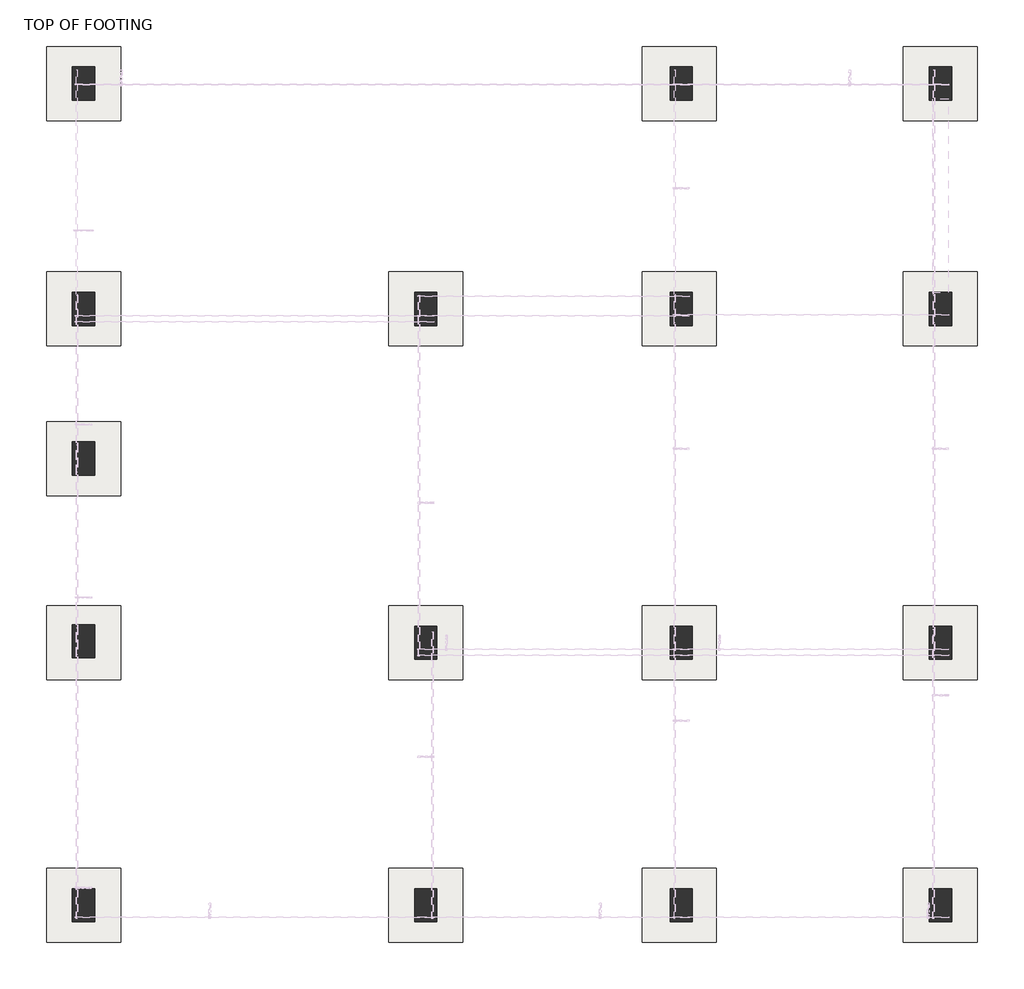
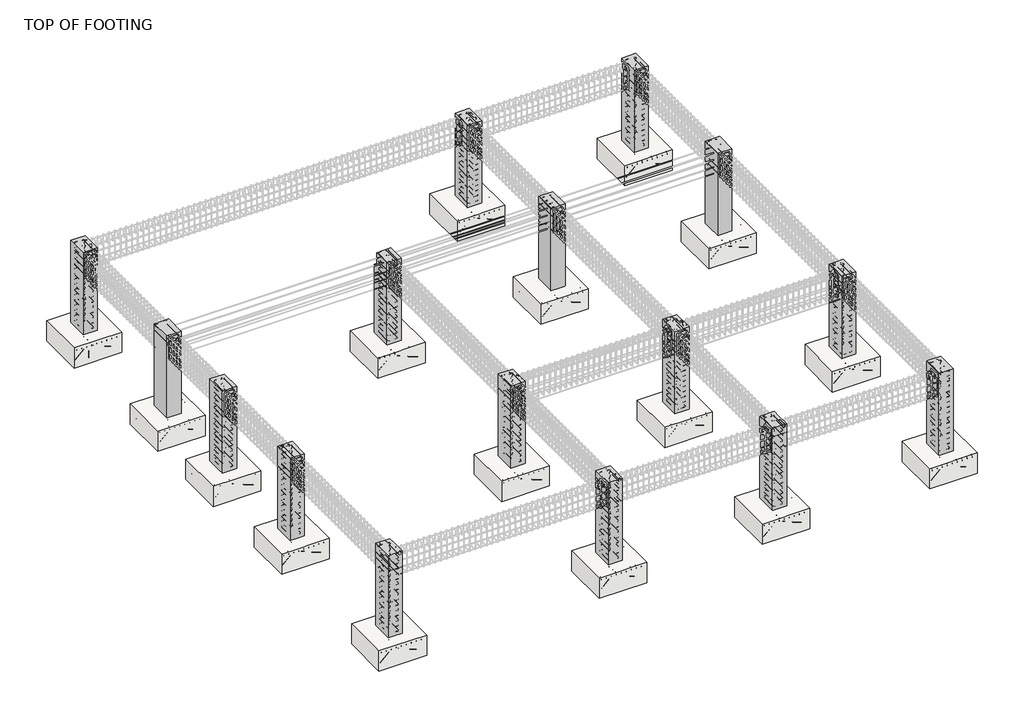
# One storey, part 1 of 13: 16 columns, 16 slabs.
"""IFC4 building model written with IfcOpenShell, lengths in millimetres."""

from ifc_helpers import new_model, si_unit, frame, origin, place, context, project, spatial, polyline, outline, extrude, faceted_brep, transform, mapped, element, save
from components import m_footing_rectangular_4c97ae35

model = new_model("IFC4")

# Units and contexts
model_context = context("Model", 3, world=origin())
ifc_project = project(units=[si_unit("LENGTHUNIT", "METRE", prefix="MILLI")], contexts=[model_context])

# Site, building, storey
site = spatial("IfcSite", under=ifc_project)
building = spatial("IfcBuilding", under=site)
storey = spatial("IfcBuildingStorey", under=building, Name="TOP OF FOOTING", Elevation=-1828.8)

# Columns
placement = place(None, origin())
element("IfcColumn", 1, ObjectType="M_Concrete-Rectangular-Column : 300 x 450mm", at=placement, inside=storey, context=model_context, shape_type="Brep", body=[
    faceted_brep([(-7173.5042006, 7072.2117918, -1828.8), (-7173.5042006, 6622.2117918, -1828.8), (-7473.5042006, 6622.2117918, -1828.8), (-7473.5042006, 7072.2117918, -1828.8), (-7173.5042006, 7072.2117918, 0.0), (-7173.5042006, 6772.2117918, 0.0), (-7173.5042006, 6622.2117918, 0.0), (-7473.5042006, 6622.2117918, 0.0), (-7473.5042006, 7072.2117918, 0.0)], [[[0, 1, 2, 3]], [[4, 5, 6, 1, 0]], [[6, 7, 2, 1]], [[7, 8, 3, 2]], [[8, 4, 0, 3]], [[4, 8, 7, 6, 5]]]),
])
element("IfcColumn", 2, ObjectType="M_Concrete-Rectangular-Column : 300 x 450mm", at=placement, inside=storey, context=model_context, shape_type="Brep", body=[
    faceted_brep([(-7173.5042006, -4034.4342236, -1828.8), (-7173.5042006, -4484.4342236, -1828.8), (-7473.5042006, -4484.4342236, -1828.8), (-7473.5042006, -4034.4342236, -1828.8), (-7173.5042006, -4034.4342236, 0.0), (-7173.5042006, -4184.4342236, 0.0), (-7173.5042006, -4484.4342236, 0.0), (-7473.5042006, -4484.4342236, 0.0), (-7473.5042006, -4034.4342236, 0.0)], [[[0, 1, 2, 3]], [[4, 5, 6, 1, 0]], [[6, 7, 2, 1]], [[7, 8, 3, 2]], [[8, 4, 0, 3]], [[4, 8, 7, 6, 5]]]),
])
element("IfcColumn", 3, ObjectType="M_Concrete-Rectangular-Column : 300 x 450mm", at=placement, inside=storey, context=model_context, shape_type="SweptSolid", body=[
    extrude(outline(polyline([(-7173.5042006, -466.4898401), (-7173.5042006, -916.4898401), (-7473.5042006, -916.4898401), (-7473.5042006, -466.4898401), (-7173.5042006, -466.4898401)])), frame((0.0, 0.0, -1828.8), z_axis=(0.0, 0.0, 1.0), x_axis=(1.0, 0.0, 0.0)), (0.0, 0.0, 1.0), 1828.8),
])
element("IfcColumn", 4, ObjectType="M_Concrete-Rectangular-Column : 300 x 450mm", at=placement, inside=storey, context=model_context, shape_type="SweptSolid", body=[
    extrude(outline(polyline([(-7173.5042006, 2002.0021284), (-7173.5042006, 1552.0021284), (-7473.5042006, 1552.0021284), (-7473.5042006, 2002.0021284), (-7173.5042006, 2002.0021284)])), frame((0.0, 0.0, -1828.8), z_axis=(0.0, 0.0, 1.0), x_axis=(1.0, 0.0, 0.0)), (0.0, 0.0, 1.0), 1828.8),
])
element("IfcColumn", 5, ObjectType="M_Concrete-Rectangular-Column : 300 x 450mm", at=placement, inside=storey, context=model_context, shape_type="Brep", body=[
    faceted_brep([(-7173.5042006, 4025.9486413, -1828.8), (-7173.5042006, 3575.9486413, -1828.8), (-7473.5042006, 3575.9486413, -1828.8), (-7473.5042006, 4025.9486413, -1828.8), (-7173.5042006, 4025.9486413, 0.0), (-7173.5042006, 3950.9486413, 0.0), (-7173.5042006, 3650.9486413, 0.0), (-7173.5042006, 3575.9486413, 0.0), (-7473.5042006, 3575.9486413, 0.0), (-7473.5042006, 4025.9486413, 0.0)], [[[0, 1, 2, 3]], [[4, 5, 6, 7, 1, 0]], [[7, 8, 2, 1]], [[8, 9, 3, 2]], [[9, 4, 0, 3]], [[4, 9, 8, 7, 6, 5]]]),
])
element("IfcColumn", 6, ObjectType="M_Concrete-Rectangular-Column : 300 x 450mm", at=placement, inside=storey, context=model_context, shape_type="Brep", body=[
    faceted_brep([(-2545.7590063, 4025.9486413, -1828.8), (-2545.7590063, 3575.9486413, -1828.8), (-2845.7590063, 3575.9486413, -1828.8), (-2845.7590063, 4025.9486413, -1828.8), (-2545.7590063, 4025.9486413, -300.0), (-2545.7590063, 3950.9486413, -300.0), (-2545.7590063, 3950.9486413, 0.0), (-2545.7590063, 3650.9486413, 0.0), (-2545.7590063, 3575.9486413, 0.0), (-2845.7590063, 3575.9486413, 0.0), (-2845.7590063, 3650.9486413, 0.0), (-2845.7590063, 3950.9486413, 0.0), (-2845.7590063, 3950.9486413, -300.0), (-2845.7590063, 4025.9486413, -300.0)], [[[0, 1, 2, 3]], [[1, 0, 4, 5, 6, 7, 8]], [[2, 1, 8, 9]], [[3, 2, 9, 10, 11, 12, 13]], [[0, 3, 13, 4]], [[9, 8, 7, 6, 11, 10]], [[12, 5, 4, 13]], [[5, 12, 11, 6]]]),
])
element("IfcColumn", 7, ObjectType="M_Concrete-Rectangular-Column : 300 x 450mm", at=placement, inside=storey, context=model_context, shape_type="Brep", body=[
    faceted_brep([(906.4957994, 7072.2117918, -1828.8), (906.4957994, 6622.2117918, -1828.8), (606.4957994, 6622.2117918, -1828.8), (606.4957994, 7072.2117918, -1828.8), (906.4957994, 7072.2117918, 0.0), (906.4957994, 6772.2117918, 0.0), (906.4957994, 6622.2117918, 0.0), (906.4957994, 7072.2117918, -600.0), (606.4957994, 6622.2117918, 0.0), (606.4957994, 6772.2117918, 0.0), (606.4957994, 7072.2117918, 0.0), (606.4957994, 7072.2117918, -600.0)], [[[0, 1, 2, 3]], [[4, 5, 6, 1, 0, 7]], [[6, 8, 2, 1]], [[8, 9, 10, 11, 3, 2]], [[10, 4, 7, 0, 3, 11]], [[4, 10, 9, 8, 6, 5]]]),
])
element("IfcColumn", 8, ObjectType="M_Concrete-Rectangular-Column : 300 x 450mm", at=placement, inside=storey, context=model_context, shape_type="SweptSolid", body=[
    extrude(outline(polyline([(4410.0083683, 7072.2117918), (4410.0083683, 6622.2117918), (4110.0083683, 6622.2117918), (4110.0083683, 7072.2117918), (4410.0083683, 7072.2117918)])), frame((0.0, 0.0, -1828.8), z_axis=(0.0, 0.0, 1.0), x_axis=(1.0, 0.0, 0.0)), (0.0, 0.0, 1.0), 1828.8),
])
element("IfcColumn", 9, ObjectType="M_Concrete-Rectangular-Column : 300 x 450mm", at=placement, inside=storey, context=model_context, shape_type="Brep", body=[
    faceted_brep([(4410.0083683, -4034.4342236, -1828.8), (4410.0083683, -4484.4342236, -1828.8), (4110.0083683, -4484.4342236, -1828.8), (4110.0083683, -4034.4342236, -1828.8), (4410.0083683, -4034.4342236, 0.0), (4410.0083683, -4484.4342236, 0.0), (4110.0083683, -4484.4342236, 0.0), (4110.0083683, -4184.4342236, 0.0), (4110.0083683, -4034.4342236, 0.0)], [[[0, 1, 2, 3]], [[4, 5, 1, 0]], [[5, 6, 2, 1]], [[6, 7, 8, 3, 2]], [[8, 4, 0, 3]], [[4, 8, 7, 6, 5]]]),
])
element("IfcColumn", 10, ObjectType="M_Concrete-Rectangular-Column : 300 x 450mm", at=placement, inside=storey, context=model_context, shape_type="Brep", body=[
    faceted_brep([(4410.0083683, 4025.9486413, -1828.8), (4410.0083683, 3575.9486413, -1828.8), (4110.0083683, 3575.9486413, -1828.8), (4110.0083683, 4025.9486413, -1828.8), (4410.0083683, 4025.9486413, 0.0), (4410.0083683, 3575.9486413, 0.0), (4110.0083683, 3575.9486413, 0.0), (4110.0083683, 3650.9486413, 0.0), (4110.0083683, 4025.9486413, 0.0)], [[[0, 1, 2, 3]], [[4, 5, 1, 0]], [[5, 6, 2, 1]], [[6, 7, 8, 3, 2]], [[8, 4, 0, 3]], [[4, 8, 7, 6, 5]]]),
])
element("IfcColumn", 11, ObjectType="M_Concrete-Rectangular-Column : 300 x 450mm", at=placement, inside=storey, context=model_context, shape_type="Brep", body=[
    faceted_brep([(4410.0083683, -486.4898401, -1828.8), (4410.0083683, -936.4898401, -1828.8), (4110.0083683, -936.4898401, -1828.8), (4110.0083683, -486.4898401, -1828.8), (4410.0083683, -486.4898401, 0.0), (4410.0083683, -936.4898401, 0.0), (4110.0083683, -936.4898401, 0.0), (4110.0083683, -861.4898401, 0.0), (4110.0083683, -561.4898401, 0.0), (4110.0083683, -486.4898401, 0.0)], [[[0, 1, 2, 3]], [[4, 5, 1, 0]], [[5, 6, 2, 1]], [[6, 7, 8, 9, 3, 2]], [[9, 4, 0, 3]], [[4, 9, 8, 7, 6, 5]]]),
])
element("IfcColumn", 12, ObjectType="M_Concrete-Rectangular-Column : 300 x 450mm", at=placement, inside=storey, context=model_context, shape_type="Brep", body=[
    faceted_brep([(905.4890092, -4034.4342236, -1828.8), (905.4890092, -4484.4342236, -1828.8), (605.4890092, -4484.4342236, -1828.8), (605.4890092, -4034.4342236, -1828.8), (905.4890092, -4034.4342236, 0.0), (905.4890092, -4184.4342236, 0.0), (905.4890092, -4484.4342236, 0.0), (605.4890092, -4484.4342236, 0.0), (605.4890092, -4184.4342236, 0.0), (605.4890092, -4034.4342236, 0.0)], [[[0, 1, 2, 3]], [[4, 5, 6, 1, 0]], [[6, 7, 2, 1]], [[7, 8, 9, 3, 2]], [[9, 4, 0, 3]], [[4, 9, 8, 7, 6, 5]]]),
])
element("IfcColumn", 13, ObjectType="M_Concrete-Rectangular-Column : 300 x 450mm", at=placement, inside=storey, context=model_context, shape_type="Brep", body=[
    faceted_brep([(-2545.7590063, -4034.4342236, -1828.8), (-2545.7590063, -4484.4342236, -1828.8), (-2845.7590063, -4484.4342236, -1828.8), (-2845.7590063, -4034.4342236, -1828.8), (-2545.7590063, -4034.4342236, 0.0), (-2545.7590063, -4184.4342236, 0.0), (-2545.7590063, -4484.4342236, 0.0), (-2845.7590063, -4484.4342236, 0.0), (-2845.7590063, -4184.4342236, 0.0), (-2845.7590063, -4034.4342236, 0.0)], [[[0, 1, 2, 3]], [[4, 5, 6, 1, 0]], [[6, 7, 2, 1]], [[7, 8, 9, 3, 2]], [[9, 4, 0, 3]], [[4, 9, 8, 7, 6, 5]]]),
])
element("IfcColumn", 14, ObjectType="M_Concrete-Rectangular-Column : 300 x 450mm", at=placement, inside=storey, context=model_context, shape_type="Brep", body=[
    faceted_brep([(905.4890092, 4025.9486413, -1828.8), (905.4890092, 3575.9486413, -1828.8), (605.4890092, 3575.9486413, -1828.8), (605.4890092, 4025.9486413, -1828.8), (905.4890092, 4025.9486413, 0.0), (905.4890092, 3650.9486413, 0.0), (905.4890092, 3575.9486413, 0.0), (905.4890092, 3575.9486413, -300.0), (605.4890092, 3575.9486413, 0.0), (605.4890092, 3575.9486413, -300.0), (605.4890092, 3650.9486413, 0.0), (605.4890092, 3950.9486413, 0.0), (605.4890092, 4025.9486413, 0.0)], [[[0, 1, 2, 3]], [[1, 0, 4, 5, 6, 7]], [[2, 1, 7, 6, 8, 9]], [[3, 2, 9, 8, 10, 11, 12]], [[0, 3, 12, 4]], [[8, 6, 5, 4, 12, 11, 10]]]),
])
element("IfcColumn", 15, ObjectType="M_Concrete-Rectangular-Column : 300 x 450mm", at=placement, inside=storey, context=model_context, shape_type="Brep", body=[
    faceted_brep([(905.4890092, -486.4898401, -1828.8), (905.4890092, -936.4898401, -1828.8), (605.4890092, -936.4898401, -1828.8), (605.4890092, -486.4898401, -1828.8), (905.4890092, -486.4898401, -300.0), (905.4890092, -486.4898401, 0.0), (905.4890092, -561.4898401, 0.0), (905.4890092, -861.4898401, 0.0), (905.4890092, -936.4898401, 0.0), (605.4890092, -936.4898401, 0.0), (605.4890092, -861.4898401, 0.0), (605.4890092, -561.4898401, 0.0), (605.4890092, -486.4898401, 0.0), (605.4890092, -486.4898401, -300.0)], [[[0, 1, 2, 3]], [[1, 0, 4, 5, 6, 7, 8]], [[2, 1, 8, 9]], [[3, 2, 9, 10, 11, 12, 13]], [[0, 3, 13, 12, 5, 4]], [[9, 8, 7, 6, 5, 12, 11, 10]]]),
])
element("IfcColumn", 16, ObjectType="M_Concrete-Rectangular-Column : 300 x 450mm", at=placement, inside=storey, context=model_context, shape_type="Brep", body=[
    faceted_brep([(-2545.7590063, -486.4898401, -1828.8), (-2545.7590063, -936.4898401, -1828.8), (-2845.7590063, -936.4898401, -1828.8), (-2845.7590063, -486.4898401, -1828.8), (-2545.7590063, -486.4898401, 0.0), (-2545.7590063, -561.4898401, 0.0), (-2545.7590063, -861.4898401, 0.0), (-2545.7590063, -936.4898401, 0.0), (-2845.7590063, -936.4898401, 0.0), (-2845.7590063, -486.4898401, 0.0)], [[[0, 1, 2, 3]], [[4, 5, 6, 7, 1, 0]], [[7, 8, 2, 1]], [[8, 9, 3, 2]], [[9, 4, 0, 3]], [[4, 9, 8, 7, 6, 5]]]),
])

# Slabs
m_footing_rectangular_shape = m_footing_rectangular_4c97ae35(model_context)
element("IfcSlab", 17, ObjectType="M_Footing-Rectangular", at=placement, inside=storey, context=model_context, shape_type="MappedRepresentation", body=[
    mapped(m_footing_rectangular_shape, transform((-7323.5042006, 6847.2117918, -1828.8), x_axis=(1.0, 0.0, 0.0), y_axis=(0.0, 1.0, 0.0), z_axis=(0.0, 0.0, 1.0))),
])
element("IfcSlab", 18, ObjectType="M_Footing-Rectangular", at=placement, inside=storey, context=model_context, shape_type="MappedRepresentation", body=[
    mapped(m_footing_rectangular_shape, transform((4260.0083683, 6847.2117918, -1828.8), x_axis=(1.0, 0.0, 0.0), y_axis=(0.0, 1.0, 0.0), z_axis=(0.0, 0.0, 1.0))),
])
element("IfcSlab", 19, ObjectType="M_Footing-Rectangular", at=placement, inside=storey, context=model_context, shape_type="MappedRepresentation", body=[
    mapped(m_footing_rectangular_shape, transform((730.4890092, 6847.2117918, -1828.8), x_axis=(1.0, 0.0, 0.0), y_axis=(0.0, 1.0, 0.0), z_axis=(0.0, 0.0, 1.0))),
])
element("IfcSlab", 20, ObjectType="M_Footing-Rectangular", at=placement, inside=storey, context=model_context, shape_type="MappedRepresentation", body=[
    mapped(m_footing_rectangular_shape, transform((-7323.5042006, 3800.9486413, -1828.8), x_axis=(1.0, 0.0, 0.0), y_axis=(0.0, 1.0, 0.0), z_axis=(0.0, 0.0, 1.0))),
])
element("IfcSlab", 21, ObjectType="M_Footing-Rectangular", at=placement, inside=storey, context=model_context, shape_type="MappedRepresentation", body=[
    mapped(m_footing_rectangular_shape, transform((730.4890092, 3800.9486413, -1828.8), x_axis=(1.0, 0.0, 0.0), y_axis=(0.0, 1.0, 0.0), z_axis=(0.0, 0.0, 1.0))),
])
element("IfcSlab", 22, ObjectType="M_Footing-Rectangular", at=placement, inside=storey, context=model_context, shape_type="MappedRepresentation", body=[
    mapped(m_footing_rectangular_shape, transform((4260.0083683, 3800.9486413, -1828.8), x_axis=(1.0, 0.0, 0.0), y_axis=(0.0, 1.0, 0.0), z_axis=(0.0, 0.0, 1.0))),
])
element("IfcSlab", 23, ObjectType="M_Footing-Rectangular", at=placement, inside=storey, context=model_context, shape_type="MappedRepresentation", body=[
    mapped(m_footing_rectangular_shape, transform((-7323.5042006, -4259.4342236, -1828.8), x_axis=(1.0, 0.0, 0.0), y_axis=(0.0, 1.0, 0.0), z_axis=(0.0, 0.0, 1.0))),
])
element("IfcSlab", 24, ObjectType="M_Footing-Rectangular", at=placement, inside=storey, context=model_context, shape_type="MappedRepresentation", body=[
    mapped(m_footing_rectangular_shape, transform((4260.0083683, -4259.4342236, -1828.8), x_axis=(1.0, 0.0, 0.0), y_axis=(0.0, 1.0, 0.0), z_axis=(0.0, 0.0, 1.0))),
])
element("IfcSlab", 25, ObjectType="M_Footing-Rectangular", at=placement, inside=storey, context=model_context, shape_type="MappedRepresentation", body=[
    mapped(m_footing_rectangular_shape, transform((-2695.7590063, 3800.9486413, -1828.8), x_axis=(1.0, 0.0, 0.0), y_axis=(0.0, 1.0, 0.0), z_axis=(0.0, 0.0, 1.0))),
])
element("IfcSlab", 26, ObjectType="M_Footing-Rectangular", at=placement, inside=storey, context=model_context, shape_type="MappedRepresentation", body=[
    mapped(m_footing_rectangular_shape, transform((-7323.5042006, -711.4898401, -1828.8), x_axis=(1.0, 0.0, 0.0), y_axis=(0.0, 1.0, 0.0), z_axis=(0.0, 0.0, 1.0))),
])
element("IfcSlab", 27, ObjectType="M_Footing-Rectangular", at=placement, inside=storey, context=model_context, shape_type="MappedRepresentation", body=[
    mapped(m_footing_rectangular_shape, transform((-2695.7590063, -711.4898401, -1828.8), x_axis=(1.0, 0.0, 0.0), y_axis=(0.0, 1.0, 0.0), z_axis=(0.0, 0.0, 1.0))),
])
element("IfcSlab", 28, ObjectType="M_Footing-Rectangular", at=placement, inside=storey, context=model_context, shape_type="MappedRepresentation", body=[
    mapped(m_footing_rectangular_shape, transform((730.4890092, -711.4898401, -1828.8), x_axis=(1.0, 0.0, 0.0), y_axis=(0.0, 1.0, 0.0), z_axis=(0.0, 0.0, 1.0))),
])
element("IfcSlab", 29, ObjectType="M_Footing-Rectangular", at=placement, inside=storey, context=model_context, shape_type="MappedRepresentation", body=[
    mapped(m_footing_rectangular_shape, transform((-2695.7590063, -4259.4342236, -1828.8), x_axis=(1.0, 0.0, 0.0), y_axis=(0.0, 1.0, 0.0), z_axis=(0.0, 0.0, 1.0))),
])
element("IfcSlab", 30, ObjectType="M_Footing-Rectangular", at=placement, inside=storey, context=model_context, shape_type="MappedRepresentation", body=[
    mapped(m_footing_rectangular_shape, transform((730.4890092, -4259.4342236, -1828.8), x_axis=(1.0, 0.0, 0.0), y_axis=(0.0, 1.0, 0.0), z_axis=(0.0, 0.0, 1.0))),
])
element("IfcSlab", 31, ObjectType="M_Footing-Rectangular", at=placement, inside=storey, context=model_context, shape_type="MappedRepresentation", body=[
    mapped(m_footing_rectangular_shape, transform((4260.0083683, -711.4898401, -1828.8), x_axis=(1.0, 0.0, 0.0), y_axis=(0.0, 1.0, 0.0), z_axis=(0.0, 0.0, 1.0))),
])
element("IfcSlab", 32, ObjectType="M_Footing-Rectangular", at=placement, inside=storey, context=model_context, shape_type="MappedRepresentation", body=[
    mapped(m_footing_rectangular_shape, transform((-7323.5042006, 1777.0021284, -1828.8), x_axis=(1.0, 0.0, 0.0), y_axis=(0.0, 1.0, 0.0), z_axis=(0.0, 0.0, 1.0))),
])

save(model, "model.ifc")

# Revit data of these elements
# Grids (mm)
#   "A": line (-7323.504, -6697.426) -> (-7323.504, 10728.766)
#   "B": line (-3923.504, -6697.426) -> (-3923.504, 10728.766)
#   "C": line (-2695.759, -6697.426) -> (-2695.759, 10728.766)
#   "D": line (730.489, -6697.426) -> (730.489, 10728.766)
#   "E": line (4260.008, -6697.426) -> (4260.008, 10728.766)
#   "1": line (-8810.13, 6847.212) -> (4958.96, 6847.212)
#   "2": line (-8810.13, 3800.949) -> (4369.257, 3800.949)
#   "3": line (-8810.13, 1777.002) -> (4314.566, 1777.002)
#   "4": line (-8810.13, -711.49) -> (4823.837, -711.49)
#   "5": line (-9513.207, -1231.49) -> (4823.837, -1231.49)
#   "6": line (-8810.13, -3259.434) -> (4823.837, -3259.434)
#   "7": line (-8810.13, -4259.434) -> (4823.837, -4259.434)
# Type "M_Concrete-Rectangular-Column : 300 x 450mm"
#   b = 300 mm
#   h = 450 mm
#   Structural Material [instance default] = Concrete, Cast-in-Place gray
# Type "M_Footing-Rectangular"
#   Width = 1000 mm
#   Length = 1000 mm
#   Foundation Thickness = 450 mm
#   Structural Material [instance default] = Concrete, Cast-in-Place gray
#   Assembly Code = ""
# Elements 1, 2, 3, 4, 5, 6, 7, 8, 9, 10, 11, 12, 13, 14, 15, 16 (IfcColumn, "M_Concrete-Rectangular-Column : 300 x 450mm")
#   Structural Material = Concrete, Cast-in-Place gray
#   Phase Created = New Construction
#   Materials on its faces: "Concrete, Cast-in-Place gray"
# Elements 17, 18, 19, 20, 21, 22, 23, 24, 25, 26, 27, 28, 29, 30, 31, 32 (IfcSlab, "M_Footing-Rectangular")
#   Structural Material = Concrete, Cast-in-Place gray
#   Phase Created = New Construction
#   Materials on its faces: "Concrete, Cast-in-Place gray"
# Materials
#   "Concrete, Cast-in-Place gray": class "Concrete", colour RGB 192 192 192, transparency 0, Description = "Cast-in-place concrete", Cost = 0
